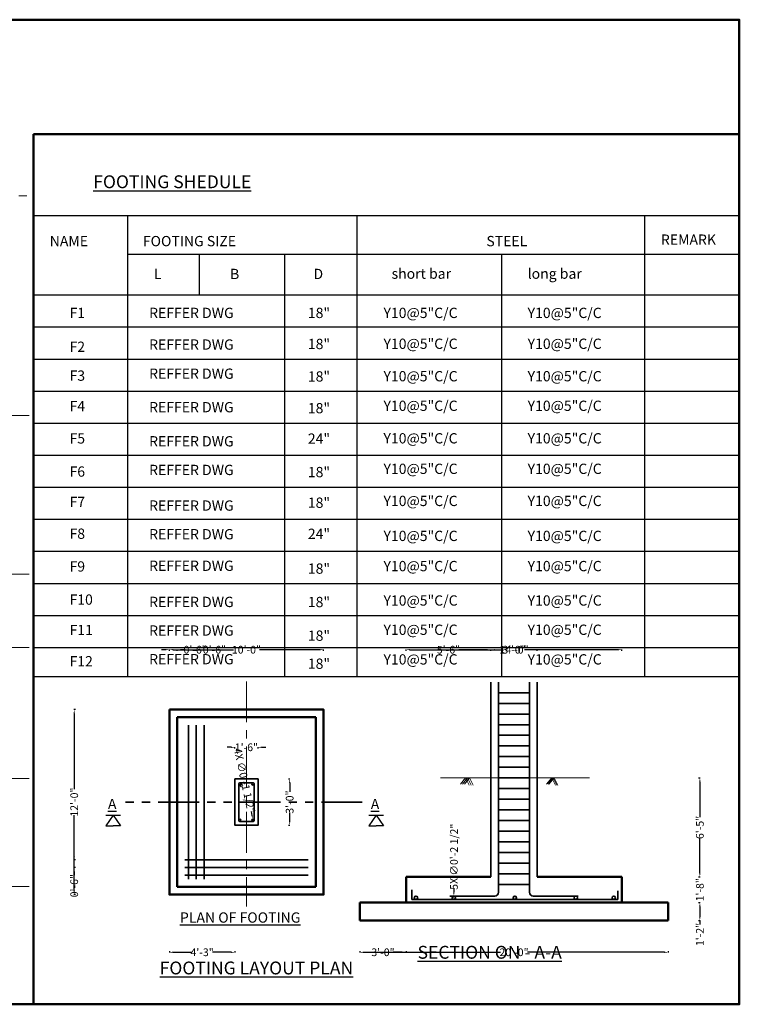
# Model space of a CAD drawing. Units: inches. Extents: x -114 to 953, y -626 to 140.
# Tile 3 of 3: x 393 to 953, y -626 to 140. Entities that reach past the tile are written whole.
import ezdxf

# ---------------------------------------------------------------- set-up
doc = ezdxf.new("R2010")
doc.units = ezdxf.units.IN
doc.header["$MEASUREMENT"] = 0
doc.linetypes.add('CENTER', pattern=[50.8, 31.75, -6.35, 6.35, -6.35])
doc.linetypes.add('PHANTOM', pattern=[63.5, 31.75, -6.35, 6.35, -6.35, 6.35, -6.35])
for name, color, linetype, lineweight in [('C-TOPO', 8, 'Continuous', 18), ('S-ANNO-DIMS', 2, 'Continuous', 25), ('S-ANNO-SCHD', 7, 'Continuous', 25), ('S-ANNO-SYMB', 3, 'Continuous', 25), ('S-ANNO-TEXT', 3, 'Continuous', 25), ('S-ANNO-TTLB', 7, 'Continuous', 50), ('S-COLS', 4, 'Continuous', 35), ('S-FNDN', 7, 'Continuous', 50), ('S-GRID', 1, 'CENTER', 18), ('S-REIN', 1, 'Continuous', 35), ('S-SECT', 6, 'PHANTOM', 35)]:
    doc.layers.add(name, color=color, linetype=linetype, lineweight=lineweight)
doc.styles.get("Standard").update_dxf_attribs({"font": 'arial.ttf'})
doc.dimstyles.get("Standard").update_dxf_attribs({"dimtxt": 6, "dimasz": 3, "dimexe": 0.18, "dimexo": 0.0625, "dimgap": 0.09, "dimtad": 0, "dimzin": 0, "dimdsep": 46, "dimlunit": 4, "dimtxsty": 'Standard', "dimcen": 0.09, "dimclrd": 256, "dimclrt": 6, "dimadec": 0, "dimazin": 0, "dimtfac": 6, "dimtofl": 0, "dimtmove": 0, "dimatfit": 3, "dimfxl": 1, "dimfxlon": 1, "dimtolj": 1, "dimtzin": 0, "dimarcsym": 0})

# ---------------------------------------------------------------- blocks, each defined once
blk = doc.blocks.new('SECTION-MARK')
for p, q in [((664.65, -479.21), (676.15, -479.21)), ((670.4, -479.21), (664.65, -487.36)), ((670.4, -479.21), (676.15, -487.36)), ((664.65, -487.36), (670.4, -487.36)), ((676.15, -487.36), (670.4, -487.36))]:
    blk.add_line(p, q)
blk = doc.blocks.new('*D64')
at = {"layer": 'Defpoints', "color": 0, "transparency": 16777216}
for p in [(629.47, -350.34), (509.47, -396.96), (629.47, -396.96)]:
    blk.add_point(p, dxfattribs=at)
at = {"layer": 'S-ANNO-DIMS', "color": 0, "lineweight": -2, "transparency": 16777216}
for p, q in [((509.47, -351.34), (509.47, -350.16)), ((629.47, -351.34), (629.47, -350.16))]:
    blk.add_line(p, q, dxfattribs=at)
at = {"layer": 'S-ANNO-DIMS', "lineweight": -2, "transparency": 16777216}
for p, q in [((512.47, -350.34), (559.36, -350.34)), ((626.47, -350.34), (579.58, -350.34))]:
    blk.add_line(p, q, dxfattribs=at)
at = {"layer": 'S-ANNO-DIMS', "transparency": 16777216}
for points in [[(512.47, -349.84), (512.47, -350.84), (509.47, -350.34)], [(626.47, -349.84), (626.47, -350.84), (629.47, -350.34)]]:
    blk.add_solid(points, dxfattribs=at)
at = {"layer": 'S-ANNO-DIMS', "color": 6, "transparency": 16777216, "insert": (569.47, -350.34), "char_height": 6, "attachment_point": 5}
blk.add_mtext('\\A1;10\'-0"', dxfattribs=at)
blk = doc.blocks.new('*D65')
at = {"layer": 'Defpoints', "color": 0, "transparency": 16777216}
for p in [(509.47, -396.96), (435.43, -540.96), (509.47, -540.96)]:
    blk.add_point(p, dxfattribs=at)
at = {"layer": 'S-ANNO-DIMS', "color": 0, "lineweight": -2, "transparency": 16777216}
for p, q in [((436.43, -396.96), (435.25, -396.96)), ((436.43, -540.96), (435.25, -540.96))]:
    blk.add_line(p, q, dxfattribs=at)
at = {"layer": 'S-ANNO-DIMS', "lineweight": -2, "transparency": 16777216}
for p, q in [((435.43, -399.96), (435.43, -458.85)), ((435.43, -537.96), (435.43, -479.07))]:
    blk.add_line(p, q, dxfattribs=at)
at = {"layer": 'S-ANNO-DIMS', "transparency": 16777216}
for points in [[(434.93, -399.96), (435.93, -399.96), (435.43, -396.96)], [(434.93, -537.96), (435.93, -537.96), (435.43, -540.96)]]:
    blk.add_solid(points, dxfattribs=at)
at = {"layer": 'S-ANNO-DIMS', "color": 6, "transparency": 16777216, "insert": (435.43, -468.96), "char_height": 6, "attachment_point": 5, "rotation": 90}
blk.add_mtext('\\A1;12\'-0"', dxfattribs=at)
blk = doc.blocks.new('*D66')
at = {"layer": 'Defpoints', "color": 0, "transparency": 16777216}
for p in [(515.47, -350.34), (509.47, -396.96), (515.47, -402.96)]:
    blk.add_point(p, dxfattribs=at)
at = {"layer": 'S-ANNO-DIMS', "lineweight": -2, "transparency": 16777216}
for p, q in [((506.47, -350.34), (503.47, -350.34)), ((518.47, -350.34), (521.47, -350.34))]:
    blk.add_line(p, q, dxfattribs=at)
at = {"layer": 'S-ANNO-DIMS', "color": 0, "lineweight": -2, "transparency": 16777216}
for p, q in [((509.47, -351.34), (509.47, -350.16)), ((515.47, -351.34), (515.47, -350.16))]:
    blk.add_line(p, q, dxfattribs=at)
at = {"layer": 'S-ANNO-DIMS', "transparency": 16777216}
for points in [[(506.47, -349.84), (506.47, -350.84), (509.47, -350.34)], [(518.47, -349.84), (518.47, -350.84), (515.47, -350.34)]]:
    blk.add_solid(points, dxfattribs=at)
at = {"layer": 'S-ANNO-DIMS', "color": 6, "transparency": 16777216, "insert": (529.54, -350.34), "char_height": 6, "attachment_point": 5}
blk.add_mtext('\\A1;0\'-6"', dxfattribs=at)
blk = doc.blocks.new('*D67')
at = {"layer": 'Defpoints', "color": 0, "transparency": 16777216}
for p in [(578.470542, -426.309234), (560.470542, -450.959234), (578.470542, -450.959234)]:
    blk.add_point(p, dxfattribs=at)
at = {"layer": 'S-ANNO-DIMS', "lineweight": -2, "transparency": 16777216}
for p, q in [((557.470542, -426.309234), (554.470542, -426.309234)), ((581.470542, -426.309234), (584.470542, -426.309234))]:
    blk.add_line(p, q, dxfattribs=at)
at = {"layer": 'S-ANNO-DIMS', "color": 0, "lineweight": -2, "transparency": 16777216}
for p, q in [((560.470542, -427.309234), (560.470542, -426.129234)), ((578.470542, -427.309234), (578.470542, -426.129234))]:
    blk.add_line(p, q, dxfattribs=at)
at = {"layer": 'S-ANNO-DIMS', "transparency": 16777216}
for points in [[(557.470542, -425.809234), (557.470542, -426.809234), (560.470542, -426.309234)], [(581.470542, -425.809234), (581.470542, -426.809234), (578.470542, -426.309234)]]:
    blk.add_solid(points, dxfattribs=at)
at = {"layer": 'S-ANNO-DIMS', "color": 6, "transparency": 16777216, "insert": (569.470542, -426.309234), "char_height": 6, "attachment_point": 5}
blk.add_mtext('\\A1;1\'-6"', dxfattribs=at)
blk = doc.blocks.new('*D68')
at = {"layer": 'Defpoints', "color": 0, "transparency": 16777216}
for p in [(578.47, -450.96), (578.47, -486.96), (603.12, -486.96)]:
    blk.add_point(p, dxfattribs=at)
at = {"layer": 'S-ANNO-DIMS', "color": 0, "lineweight": -2, "transparency": 16777216}
for p, q in [((602.12, -450.96), (603.3, -450.96)), ((602.12, -486.96), (603.3, -486.96))]:
    blk.add_line(p, q, dxfattribs=at)
at = {"layer": 'S-ANNO-DIMS', "lineweight": -2, "transparency": 16777216}
for p, q in [((603.12, -453.96), (603.12, -460.9)), ((603.12, -483.96), (603.12, -477.02))]:
    blk.add_line(p, q, dxfattribs=at)
at = {"layer": 'S-ANNO-DIMS', "transparency": 16777216}
for points in [[(602.62, -453.96), (603.62, -453.96), (603.12, -450.96)], [(602.62, -483.96), (603.62, -483.96), (603.12, -486.96)]]:
    blk.add_solid(points, dxfattribs=at)
at = {"layer": 'S-ANNO-DIMS', "color": 6, "transparency": 16777216, "insert": (603.12, -468.96), "char_height": 6, "attachment_point": 5, "rotation": 90}
blk.add_mtext('\\A1;3\'-0"', dxfattribs=at)
blk = doc.blocks.new('*D69')
at = {"layer": 'Defpoints', "color": 0, "transparency": 16777216}
for p in [(560.47, -486.96), (509.47, -540.96), (560.47, -585.86)]:
    blk.add_point(p, dxfattribs=at)
at = {"layer": 'S-ANNO-DIMS', "color": 0, "lineweight": -2, "transparency": 16777216}
for p, q in [((509.47, -584.86), (509.47, -586.04)), ((560.47, -584.86), (560.47, -586.04))]:
    blk.add_line(p, q, dxfattribs=at)
at = {"layer": 'S-ANNO-DIMS', "lineweight": -2, "transparency": 16777216}
for p, q in [((512.47, -585.86), (526.79, -585.86)), ((557.47, -585.86), (543.16, -585.86))]:
    blk.add_line(p, q, dxfattribs=at)
at = {"layer": 'S-ANNO-DIMS', "transparency": 16777216}
for points in [[(512.47, -585.36), (512.47, -586.36), (509.47, -585.86)], [(557.47, -585.36), (557.47, -586.36), (560.47, -585.86)]]:
    blk.add_solid(points, dxfattribs=at)
at = {"layer": 'S-ANNO-DIMS', "color": 6, "transparency": 16777216, "insert": (534.97, -585.86), "char_height": 6, "attachment_point": 5}
blk.add_mtext('\\A1;4\'-3"', dxfattribs=at)
blk = doc.blocks.new('*D70')
at = {"layer": 'Defpoints', "color": 0, "transparency": 16777216}
for p in [(530.47, -350.34), (524.47, -408.96), (530.47, -408.96)]:
    blk.add_point(p, dxfattribs=at)
at = {"layer": 'S-ANNO-DIMS', "lineweight": -2, "transparency": 16777216}
for p, q in [((521.47, -350.34), (518.47, -350.34)), ((533.47, -350.34), (536.47, -350.34))]:
    blk.add_line(p, q, dxfattribs=at)
at = {"layer": 'S-ANNO-DIMS', "color": 0, "lineweight": -2, "transparency": 16777216}
for p, q in [((524.47, -351.34), (524.47, -350.16)), ((530.47, -351.34), (530.47, -350.16))]:
    blk.add_line(p, q, dxfattribs=at)
at = {"layer": 'S-ANNO-DIMS', "transparency": 16777216}
for points in [[(521.47, -349.84), (521.47, -350.84), (524.47, -350.34)], [(533.47, -349.84), (533.47, -350.84), (530.47, -350.34)]]:
    blk.add_solid(points, dxfattribs=at)
at = {"layer": 'S-ANNO-DIMS', "color": 6, "transparency": 16777216, "insert": (544.54, -350.34), "char_height": 6, "attachment_point": 5}
blk.add_mtext('\\A1;0\'-6"', dxfattribs=at)
blk = doc.blocks.new('*D71')
at = {"layer": 'Defpoints', "color": 0, "transparency": 16777216}
for p in [(435.43, -519.96), (521.47, -513.96), (521.47, -519.96)]:
    blk.add_point(p, dxfattribs=at)
at = {"layer": 'S-ANNO-DIMS', "lineweight": -2, "transparency": 16777216}
for p, q in [((435.43, -510.96), (435.43, -507.96)), ((435.43, -522.96), (435.43, -525.96))]:
    blk.add_line(p, q, dxfattribs=at)
at = {"layer": 'S-ANNO-DIMS', "color": 0, "lineweight": -2, "transparency": 16777216}
for p, q in [((436.43, -513.96), (435.25, -513.96)), ((436.43, -519.96), (435.25, -519.96))]:
    blk.add_line(p, q, dxfattribs=at)
at = {"layer": 'S-ANNO-DIMS', "transparency": 16777216}
for points in [[(434.93, -510.96), (435.93, -510.96), (435.43, -513.96)], [(434.93, -522.96), (435.93, -522.96), (435.43, -519.96)]]:
    blk.add_solid(points, dxfattribs=at)
at = {"layer": 'S-ANNO-DIMS', "color": 6, "transparency": 16777216, "insert": (435.43, -534.02), "char_height": 6, "attachment_point": 5, "rotation": 90}
blk.add_mtext('\\A1;0\'-6"', dxfattribs=at)
blk = doc.blocks.new('*D72')
at = {"layer": 'Defpoints', "color": 0, "transparency": 16777216}
for p in [(657.72, -561.21), (897.72, -561.21), (897.72, -585.86)]:
    blk.add_point(p, dxfattribs=at)
at = {"layer": 'S-ANNO-DIMS', "color": 0, "lineweight": -2, "transparency": 16777216}
for p, q in [((657.72, -584.86), (657.72, -586.04)), ((897.72, -584.86), (897.72, -586.04))]:
    blk.add_line(p, q, dxfattribs=at)
at = {"layer": 'S-ANNO-DIMS', "lineweight": -2, "transparency": 16777216}
for p, q in [((660.72, -585.86), (767.27, -585.86)), ((894.72, -585.86), (788.17, -585.86))]:
    blk.add_line(p, q, dxfattribs=at)
at = {"layer": 'S-ANNO-DIMS', "transparency": 16777216}
for points in [[(660.72, -585.36), (660.72, -586.36), (657.72, -585.86)], [(894.72, -585.36), (894.72, -586.36), (897.72, -585.86)]]:
    blk.add_solid(points, dxfattribs=at)
at = {"layer": 'S-ANNO-DIMS', "color": 6, "transparency": 16777216, "insert": (777.72, -585.86), "char_height": 6, "attachment_point": 5}
blk.add_mtext('\\A1;20\'-0"', dxfattribs=at)
blk = doc.blocks.new('*D73')
at = {"layer": 'Defpoints', "color": 0, "transparency": 16777216}
for p in [(657.72, -547.21), (693.72, -547.21), (693.72, -585.86)]:
    blk.add_point(p, dxfattribs=at)
at = {"layer": 'S-ANNO-DIMS', "color": 0, "lineweight": -2, "transparency": 16777216}
for p, q in [((657.72, -584.86), (657.72, -586.04)), ((693.72, -584.86), (693.72, -586.04))]:
    blk.add_line(p, q, dxfattribs=at)
at = {"layer": 'S-ANNO-DIMS', "lineweight": -2, "transparency": 16777216}
for p, q in [((660.72, -585.86), (667.66, -585.86)), ((690.72, -585.86), (683.78, -585.86))]:
    blk.add_line(p, q, dxfattribs=at)
at = {"layer": 'S-ANNO-DIMS', "transparency": 16777216}
for points in [[(660.72, -585.36), (660.72, -586.36), (657.72, -585.86)], [(690.72, -585.36), (690.72, -586.36), (693.72, -585.86)]]:
    blk.add_solid(points, dxfattribs=at)
at = {"layer": 'S-ANNO-DIMS', "color": 6, "transparency": 16777216, "insert": (675.72, -585.86), "char_height": 6, "attachment_point": 5}
blk.add_mtext('\\A1;3\'-0"', dxfattribs=at)
blk = doc.blocks.new('*D74')
at = {"layer": 'Defpoints', "color": 0, "transparency": 16777216}
for p in [(861.72, -350.34), (693.72, -527.21), (861.72, -527.21)]:
    blk.add_point(p, dxfattribs=at)
at = {"layer": 'S-ANNO-DIMS', "color": 0, "lineweight": -2, "transparency": 16777216}
for p, q in [((693.72, -351.34), (693.72, -350.16)), ((861.72, -351.34), (861.72, -350.16))]:
    blk.add_line(p, q, dxfattribs=at)
at = {"layer": 'S-ANNO-DIMS', "lineweight": -2, "transparency": 16777216}
for p, q in [((696.72, -350.34), (767.61, -350.34)), ((858.72, -350.34), (787.83, -350.34))]:
    blk.add_line(p, q, dxfattribs=at)
at = {"layer": 'S-ANNO-DIMS', "transparency": 16777216}
for points in [[(696.72, -349.84), (696.72, -350.84), (693.72, -350.34)], [(858.72, -349.84), (858.72, -350.84), (861.72, -350.34)]]:
    blk.add_solid(points, dxfattribs=at)
at = {"layer": 'S-ANNO-DIMS', "color": 6, "transparency": 16777216, "insert": (777.72, -350.34), "char_height": 6, "attachment_point": 5}
blk.add_mtext('\\A1;14\'-0"', dxfattribs=at)
blk = doc.blocks.new('*D75')
at = {"layer": 'Defpoints', "color": 0, "transparency": 16777216}
for p in [(897.72, -547.21), (897.72, -561.21), (922.37, -561.21)]:
    blk.add_point(p, dxfattribs=at)
at = {"layer": 'S-ANNO-DIMS', "color": 0, "lineweight": -2, "transparency": 16777216}
for p, q in [((921.37, -547.21), (922.55, -547.21)), ((921.37, -561.21), (922.55, -561.21))]:
    blk.add_line(p, q, dxfattribs=at)
at = {"layer": 'S-ANNO-DIMS', "lineweight": -2, "transparency": 16777216}
for p, q in [((922.37, -550.21), (922.37, -558.21)), ((922.37, -561.21), (922.37, -564.21))]:
    blk.add_line(p, q, dxfattribs=at)
at = {"layer": 'S-ANNO-DIMS', "transparency": 16777216}
for points in [[(921.87, -550.21), (922.87, -550.21), (922.37, -547.21)], [(921.87, -558.21), (922.87, -558.21), (922.37, -561.21)]]:
    blk.add_solid(points, dxfattribs=at)
at = {"layer": 'S-ANNO-DIMS', "color": 6, "transparency": 16777216, "insert": (922.37, -571.99), "char_height": 6, "attachment_point": 5, "rotation": 90}
blk.add_mtext('\\A1;1\'-2"', dxfattribs=at)
blk = doc.blocks.new('*D76')
at = {"layer": 'Defpoints', "color": 0, "transparency": 16777216}
for p in [(861.721337, -527.205723), (861.721337, -547.205723), (922.371337, -547.205723)]:
    blk.add_point(p, dxfattribs=at)
at = {"layer": 'S-ANNO-DIMS', "color": 0, "lineweight": -2, "transparency": 16777216}
for p, q in [((921.371337, -527.205723), (922.551337, -527.205723)), ((921.371337, -547.205723), (922.551337, -547.205723))]:
    blk.add_line(p, q, dxfattribs=at)
at = {"layer": 'S-ANNO-DIMS', "lineweight": -2, "transparency": 16777216}
for p, q in [((922.371337, -524.205723), (922.371337, -521.205723)), ((922.371337, -550.205723), (922.371337, -553.205723))]:
    blk.add_line(p, q, dxfattribs=at)
at = {"layer": 'S-ANNO-DIMS', "transparency": 16777216}
for points in [[(921.871337, -524.205723), (922.871337, -524.205723), (922.371337, -527.205723)], [(921.871337, -550.205723), (922.871337, -550.205723), (922.371337, -547.205723)]]:
    blk.add_solid(points, dxfattribs=at)
at = {"layer": 'S-ANNO-DIMS', "color": 6, "transparency": 16777216, "insert": (922.371337, -537.205723), "char_height": 6, "attachment_point": 5, "rotation": 90}
blk.add_mtext('\\A1;1\'-8"', dxfattribs=at)
blk = doc.blocks.new('*D77')
at = {"layer": 'Defpoints', "color": 0, "transparency": 16777216}
for p in [(795.72, -350.34), (759.72, -375.52), (795.72, -375.52)]:
    blk.add_point(p, dxfattribs=at)
at = {"layer": 'S-ANNO-DIMS', "color": 0, "lineweight": -2, "transparency": 16777216}
for p, q in [((759.72, -351.34), (759.72, -350.16)), ((795.72, -351.34), (795.72, -350.16))]:
    blk.add_line(p, q, dxfattribs=at)
at = {"layer": 'S-ANNO-DIMS', "lineweight": -2, "transparency": 16777216}
for p, q in [((762.72, -350.34), (769.66, -350.34)), ((792.72, -350.34), (785.78, -350.34))]:
    blk.add_line(p, q, dxfattribs=at)
at = {"layer": 'S-ANNO-DIMS', "transparency": 16777216}
for points in [[(762.72, -349.84), (762.72, -350.84), (759.72, -350.34)], [(792.72, -349.84), (792.72, -350.84), (795.72, -350.34)]]:
    blk.add_solid(points, dxfattribs=at)
at = {"layer": 'S-ANNO-DIMS', "color": 6, "transparency": 16777216, "insert": (777.72, -350.34), "char_height": 6, "attachment_point": 5}
blk.add_mtext('\\A1;3\'-0"', dxfattribs=at)
blk = doc.blocks.new('*D78')
at = {"layer": 'Defpoints', "color": 0, "transparency": 16777216}
for p in [(759.72, -350.34), (693.72, -527.21), (759.72, -527.21)]:
    blk.add_point(p, dxfattribs=at)
at = {"layer": 'S-ANNO-DIMS', "color": 0, "lineweight": -2, "transparency": 16777216}
for p, q in [((693.72, -351.34), (693.72, -350.16)), ((759.72, -351.34), (759.72, -350.16))]:
    blk.add_line(p, q, dxfattribs=at)
at = {"layer": 'S-ANNO-DIMS', "lineweight": -2, "transparency": 16777216}
for p, q in [((696.72, -350.34), (718.66, -350.34)), ((756.72, -350.34), (734.79, -350.34))]:
    blk.add_line(p, q, dxfattribs=at)
at = {"layer": 'S-ANNO-DIMS', "transparency": 16777216}
for points in [[(696.72, -349.84), (696.72, -350.84), (693.72, -350.34)], [(756.72, -349.84), (756.72, -350.84), (759.72, -350.34)]]:
    blk.add_solid(points, dxfattribs=at)
at = {"layer": 'S-ANNO-DIMS', "color": 6, "transparency": 16777216, "insert": (726.72, -350.34), "char_height": 6, "attachment_point": 5}
blk.add_mtext('\\A1;5\'-6"', dxfattribs=at)
blk = doc.blocks.new('*D79')
at = {"layer": 'Defpoints', "color": 0, "transparency": 16777216}
for p in [(836.59, -450.18), (861.72, -527.21), (922.37, -527.21)]:
    blk.add_point(p, dxfattribs=at)
at = {"layer": 'S-ANNO-DIMS', "color": 0, "lineweight": -2, "transparency": 16777216}
for p, q in [((921.37, -450.18), (922.55, -450.18)), ((921.37, -527.21), (922.55, -527.21))]:
    blk.add_line(p, q, dxfattribs=at)
at = {"layer": 'S-ANNO-DIMS', "lineweight": -2, "transparency": 16777216}
for p, q in [((922.37, -453.18), (922.37, -480.61)), ((922.37, -524.21), (922.37, -496.77))]:
    blk.add_line(p, q, dxfattribs=at)
at = {"layer": 'S-ANNO-DIMS', "transparency": 16777216}
for points in [[(921.87, -453.18), (922.87, -453.18), (922.37, -450.18)], [(921.87, -524.21), (922.87, -524.21), (922.37, -527.21)]]:
    blk.add_solid(points, dxfattribs=at)
at = {"layer": 'S-ANNO-DIMS', "color": 6, "transparency": 16777216, "insert": (922.37, -488.69), "char_height": 6, "attachment_point": 5, "rotation": 90}
blk.add_mtext('\\A1;6\'-5"', dxfattribs=at)
blk = doc.blocks.new('*D80')
at = {"layer": 'Defpoints', "color": 0, "transparency": 16777216}
for p in [(730.9, -542.07), (730.89, -544.71)]:
    blk.add_point(p, dxfattribs=at)
at = {"layer": 'S-ANNO-DIMS', "lineweight": -2, "transparency": 16777216}
blk.add_line((730.92, -536.07), (730.91, -539.07), dxfattribs=at)
at = {"layer": 'S-ANNO-DIMS', "color": 0, "lineweight": -2, "transparency": 16777216}
for p, q in [((730.81, -543.39), (730.99, -543.39)), ((730.9, -543.48), (730.9, -543.3))]:
    blk.add_line(p, q, dxfattribs=at)
at = {"layer": 'S-ANNO-DIMS', "transparency": 16777216}
blk.add_solid([(730.41, -539.07), (731.41, -539.08), (730.9, -542.07)], dxfattribs=at)
at = {"layer": 'S-ANNO-DIMS', "color": 6, "transparency": 16777216, "insert": (731.01, -511.47), "char_height": 6, "attachment_point": 5, "rotation": 89.79463}
blk.add_mtext('\\A1;5X ∅0\'-2 1/2"', dxfattribs=at)
blk = doc.blocks.new('*D81')
at = {"layer": 'Defpoints', "color": 0, "transparency": 16777216}
for p in [(574.42, -482.25), (574.79, -483.94)]:
    blk.add_point(p, dxfattribs=at)
at = {"layer": 'S-ANNO-DIMS', "lineweight": -2, "transparency": 16777216}
blk.add_line((573.16, -476.38), (573.79, -479.32), dxfattribs=at)
at = {"layer": 'S-ANNO-DIMS', "color": 0, "lineweight": -2, "transparency": 16777216}
for p, q in [((574.52, -483.1), (574.7, -483.1)), ((574.61, -483.19), (574.61, -483.01))]:
    blk.add_line(p, q, dxfattribs=at)
at = {"layer": 'S-ANNO-DIMS', "transparency": 16777216}
blk.add_solid([(574.28, -479.21), (573.3, -479.42), (574.42, -482.25)], dxfattribs=at)
at = {"layer": 'S-ANNO-DIMS', "color": 6, "transparency": 16777216, "insert": (567.96, -452.21), "char_height": 6, "attachment_point": 5, "rotation": 282.14454}
blk.add_mtext('\\A1;4X ∅0\'-1 1/2"', dxfattribs=at)

msp = doc.modelspace()

# ---------------------------------------------------------------- linework, layer by layer
at = {"layer": 'C-TOPO'}
for p, q in [((765.721, -450.18), (720.576, -450.18)), ((740.037, -450.18), (736.031, -454.899)), ((741.517, -450.18), (737.51, -454.899)), ((743.149, -450.18), (739.142, -454.899)), ((740.037, -450.18), (742.876, -455.899)), ((741.517, -450.18), (744.355, -455.899)), ((743.149, -450.18), (745.987, -455.899)), ((789.721, -450.18), (836.59, -450.18)), ((807.104, -450.18), (803.097, -454.899)), ((808.197, -450.18), (804.19, -454.899)), ((808.923, -450.18), (804.917, -454.899)), ((807.104, -450.18), (809.942, -455.899)), ((808.197, -450.18), (811.035, -455.899)), ((808.923, -450.18), (811.761, -455.899))]:
    msp.add_line(p, q, dxfattribs=at)
at = {"layer": 'S-ANNO-SCHD'}
for p, q in [((476.825, -12.309), (476.825, -371.554)), ((655.403, -12.309), (655.403, -371.554)), ((879.341, -12.309), (879.341, -371.554)), ((476.825, -42.59), (953.065, -42.59)), ((532.591, -42.59), (532.591, -74.219)), ((599.019, -42.59), (599.019, -371.554)), ((768.005, -42.59), (768.005, -371.554)), ((403.662, -74.219), (953.065, -74.219)), ((403.662, -99.164), (953.065, -99.164)), ((403.662, -124.109), (953.065, -124.109)), ((403.662, -149.054), (953.065, -149.054)), ((403.662, -173.999), (953.065, -173.999)), ((403.662, -198.944), (953.065, -198.944)), ((403.662, -223.889), (953.065, -223.889)), ((403.662, -248.833), (953.065, -248.833)), ((403.662, -273.778), (953.065, -273.778)), ((403.662, -298.723), (953.065, -298.723)), ((403.662, -323.668), (953.065, -323.668)), ((403.662, -348.613), (953.065, -348.613))]:
    msp.add_line(p, q, dxfattribs=at)
msp.add_lwpolyline([(953.065, -371.554), (403.662, -371.554), (403.662, -12.309), (953.065, -12.309)], dxfattribs=at)
at = {"layer": 'S-ANNO-TTLB'}
for points in [[(-86.343, 140.009), (953.065, 140.009), (953.065, -626.35), (-86.343, -626.35)], [(403.662, 50.843), (953.065, 50.843), (953.065, -626.35), (403.662, -626.35)]]:
    msp.add_lwpolyline(points, close=True, dxfattribs=at)
at = {"layer": 'S-COLS'}
for p, q in [((759.721, -527.206), (759.721, -375.516)), ((795.721, -527.206), (795.721, -375.516))]:
    msp.add_line(p, q, dxfattribs=at)
msp.add_lwpolyline([(560.471, -450.959), (578.471, -450.959), (578.471, -486.959), (560.471, -486.959)], close=True, dxfattribs=at)
at = {"layer": 'S-FNDN'}
for p, q in [((515.471, -402.959), (623.471, -402.959)), ((515.471, -534.959), (515.471, -402.959)), ((623.471, -402.959), (623.471, -534.959)), ((693.721, -547.206), (693.721, -527.206)), ((693.721, -527.206), (759.721, -527.206)), ((795.721, -527.206), (861.721, -527.206)), ((861.721, -547.206), (861.721, -527.206)), ((623.471, -534.959), (515.471, -534.959)), ((897.721, -547.206), (657.721, -547.206)), ((657.721, -547.206), (657.721, -561.206)), ((897.721, -547.206), (861.721, -547.206)), ((897.721, -556.206), (897.721, -547.206)), ((897.721, -561.206), (897.721, -556.206)), ((657.721, -561.206), (897.721, -561.206))]:
    msp.add_line(p, q, dxfattribs=at)
msp.add_lwpolyline([(509.471, -396.959), (629.471, -396.959), (629.471, -540.959), (509.471, -540.959)], close=True, dxfattribs=at)
at = {"layer": 'S-GRID'}
for p, q in [((-52.223, 2.831), (403.662, 2.831)), ((-37.867, -168.169), (403.662, -168.169)), ((-37.867, -291.669), (403.662, -291.669)), ((-37.867, -348.669), (403.662, -348.669)), ((569.471, -374.987), (569.471, -550.338)), ((-37.867, -450.669), (403.662, -450.669)), ((-37.867, -534.669), (403.662, -534.669))]:
    msp.add_line(p, q, dxfattribs=at)
at = {"layer": 'S-REIN'}
for p, q in [((765.721, -527.206), (765.721, -375.516)), ((789.721, -527.206), (789.721, -375.516)), ((765.721, -383.812), (789.721, -383.812)), ((765.721, -392.108), (789.721, -392.108)), ((765.721, -400.404), (789.721, -400.404)), ((524.471, -528.959), (524.471, -408.959)), ((530.471, -528.959), (530.471, -408.959)), ((536.471, -528.959), (536.471, -408.959)), ((765.721, -408.7), (789.721, -408.7)), ((765.721, -416.996), (789.721, -416.996)), ((765.721, -425.292), (789.721, -425.292)), ((765.721, -433.588), (789.721, -433.588)), ((765.721, -441.884), (789.721, -441.884)), ((765.721, -450.18), (789.721, -450.18)), ((563.775, -455.481), (565.66, -457.086)), ((564.938, -454.205), (566.748, -455.971)), ((765.721, -458.476), (789.721, -458.476)), ((765.721, -466.772), (789.721, -466.772)), ((765.721, -475.068), (789.721, -475.068)), ((765.721, -483.364), (789.721, -483.364)), ((765.721, -491.66), (789.721, -491.66)), ((765.721, -499.956), (789.721, -499.956)), ((765.721, -508.252), (789.721, -508.252)), ((617.471, -513.959), (521.471, -513.959)), ((617.471, -519.959), (521.471, -519.959)), ((765.721, -516.548), (789.721, -516.548)), ((617.471, -525.959), (521.471, -525.959)), ((765.721, -524.844), (789.721, -524.844)), ((765.721, -527.206), (765.721, -539.074)), ((789.721, -527.206), (789.721, -539.074)), ((765.721, -533.14), (789.721, -533.14)), ((698.218, -544.706), (698.218, -537.327)), ((762.721, -542.074), (727.691, -542.074)), ((792.721, -542.074), (827.752, -542.074)), ((858.606, -538.041), (858.606, -544.706)), ((858.606, -544.706), (698.218, -544.706))]:
    msp.add_line(p, q, dxfattribs=at)
for points in [[(563.471, -483.095), (563.471, -454.823)], [(564.335, -453.959), (574.607, -453.959)], [(575.471, -454.823), (575.471, -483.095)], [(574.607, -483.959), (564.335, -483.959)]]:
    msp.add_lwpolyline(points, dxfattribs=at)
for centre, radius in [((564.335, -454.823), 0.864), ((574.607, -454.823), 0.864), ((564.335, -483.095), 0.864), ((574.607, -483.095), 0.864), ((701.421, -543.39), 1.316), ((730.898, -543.39), 1.316), ((778.328, -543.39), 1.316), ((778.412, -543.39), 1.316), ((825.842, -543.39), 1.316), ((855.318, -543.39), 1.316)]:
    msp.add_circle(centre, radius, dxfattribs=at)
for centre, start, end in [((762.721, -539.074), 270, 0), ((792.721, -539.074), 180, 270)]:
    msp.add_arc(centre, 3, start, end, dxfattribs=at)
at = {"layer": 'S-SECT'}
msp.add_line((659.593, -468.959), (473.882, -468.959), dxfattribs=at)

# ---------------------------------------------------------------- block references
at = {"layer": 'S-ANNO-SYMB'}
for p in [(-204.57, 0), (0, 0)]:
    msp.add_blockref('SECTION-MARK', p, dxfattribs=at)

# ---------------------------------------------------------------- texts
at = {"layer": 'S-ANNO-TEXT', "attachment_point": 1}
for s, width, insert, char_height in [('{\\fArial|b1|i0|c0|p34;\\LFOOTING SHEDULE}', 171.9614, (450.242, 18.859), 10), ('{\\fArial|b1|i0|c0|p34;NAME}', 117.31259, (416.369, -28.326), 8), ('{\\fArial|b1|i0|c0|p34;FOOTING SIZE}', 117.31259, (488.85, -28.326), 8), ('{\\fArial|b1|i0|c0|p34;STEEL}', 117.31259, (756.218, -28.326), 8), ('{\\fArial|b1|i0|c0|p34;REMARK}', 117.31259, (892.058, -27.178), 8), ('{\\fArial|b1|i0|c0|p34;short bar }', 117.31259, (682.452, -53.653), 8), ('{\\fArial|b1|i0|c0|p34;long bar}', 117.31259, (788.362, -53.653), 8), ('{\\fArial|b1|i0|c0|p34;L}', 117.31259, (497.407, -53.901), 8), ('{\\fArial|b1|i0|c0|p34;B}', 117.31259, (556.713, -53.901), 8), ('{\\fArial|b1|i0|c0|p34;D}', 117.31259, (621.647, -53.901), 8), ('F1', 8, (431.793, -84.2), 8), ('REFFER DWG', 84.43388, (493.728, -84.2), 8), ('18"', 8, (617.269, -84.2), 8), ('Y10@5"C/C', 8, (676.145, -84.2), 8), ('Y10@5"C/C', 8, (788.306, -84.2), 8), ('F2', 8, (431.793, -110.554), 8), ('REFFER DWG', 84.43388, (493.728, -108.839), 8), ('18"', 8, (617.269, -108.389), 8), ('Y10@5"C/C', 8, (676.145, -108.224), 8), ('Y10@5"C/C', 8, (788.306, -108.224), 8), ('F3', 8, (431.793, -133.03), 8), ('REFFER DWG', 84.43388, (493.728, -131.514), 8), ('18"', 8, (617.269, -133.65), 8), ('Y10@5"C/C', 8, (676.145, -133.48), 8), ('Y10@5"C/C', 8, (788.306, -133.48), 8), ('F4', 8, (431.793, -156.754), 8), ('REFFER DWG', 84.43388, (493.728, -157.591), 8), ('18"', 8, (617.269, -158.341), 8), ('Y10@5"C/C', 8, (676.145, -156.497), 8), ('Y10@5"C/C', 8, (788.306, -156.497), 8), ('F5', 8, (431.793, -181.895), 8), ('24"', 8, (617.269, -182.071), 8), ('Y10@5"C/C', 8, (676.145, -181.81), 8), ('Y10@5"C/C', 8, (788.306, -181.81), 8), ('REFFER DWG', 84.43388, (493.728, -184.13), 8), ('REFFER DWG', 84.43388, (493.728, -206.427), 8), ('Y10@5"C/C', 8, (676.145, -205.554), 8), ('Y10@5"C/C', 8, (788.306, -205.554), 8), ('F6', 8, (431.793, -207.688), 8), ('18"', 8, (617.269, -208.097), 8), ('Y10@5"C/C', 8, (676.145, -230.551), 8), ('Y10@5"C/C', 8, (788.306, -230.551), 8), ('F7', 8, (431.793, -231.363), 8), ('REFFER DWG', 84.43388, (493.728, -234.153), 8), ('18"', 8, (617.269, -231.924), 8), ('F8', 8, (431.793, -256.05), 8), ('REFFER DWG', 84.43388, (493.728, -256.45), 8), ('24"', 8, (617.269, -256.139), 8), ('Y10@5"C/C', 8, (676.145, -257.766), 8), ('Y10@5"C/C', 8, (788.306, -257.766), 8), ('F9', 8, (431.793, -281.558), 8), ('REFFER DWG', 84.43388, (493.728, -281.015), 8), ('18"', 8, (617.269, -283.21), 8), ('Y10@5"C/C', 8, (676.145, -281.267), 8), ('Y10@5"C/C', 8, (788.306, -281.267), 8), ('F10', 8, (431.793, -307.351), 8), ('REFFER DWG', 84.43388, (493.728, -309.15), 8), ('18"', 8, (617.269, -309.237), 8), ('Y10@5"C/C', 8, (676.145, -308.048), 8), ('Y10@5"C/C', 8, (788.306, -308.048), 8), ('F11', 8, (431.793, -331.02), 8), ('REFFER DWG', 84.43388, (493.728, -331.447), 8), ('18"', 8, (617.269, -335.418), 8), ('Y10@5"C/C', 8, (676.145, -330.823), 8), ('Y10@5"C/C', 8, (788.306, -330.823), 8), ('F12', 8, (431.793, -355.339), 8), ('REFFER DWG', 84.43388, (493.728, -353.744), 8), ('18"', 8, (617.269, -357.234), 8), ('Y10@5"C/C', 8, (676.145, -353.877), 8), ('Y10@5"C/C', 8, (788.306, -353.877), 8), ('{\\fArial|b1|i0|c0|p34;\\LA}', 16.75606, (461.675, -466.435), 8), ('{\\fArial|b1|i0|c0|p34;\\LA}', 16.75606, (666.246, -466.435), 8), ('{\\fArial|b1|i0|c0|p34;\\LPLAN OF FOOTING}', 117.31259, (517.725, -554.805), 8), ('{\\fArial|b1|i0|c0|p34;\\LSECTION ON - A-A}', 132.49062, (702.657, -580.868), 10), ('{\\fArial|b1|i0|c0|p34;\\LFOOTING LAYOUT PLAN}', 171.9614, (501.939, -593.07), 10)]:
    msp.add_mtext_dynamic_manual_height_columns(s, width=width, gutter_width=1, heights=[0], dxfattribs=dict(at, insert=insert, char_height=char_height))

# ---------------------------------------------------------------- dimensions: what is measured, and where the dimension line sits
at = {"layer": 'S-ANNO-DIMS'}
for base, p1, p2, picture, middle in [((515.471, -350.337), (509.471, -396.959), (515.471, -402.959), '*D66', (529.535, -350.337)), ((629.471, -350.337), (509.471, -396.959), (629.471, -396.959), '*D64', (569.471, -350.337)), ((530.471, -350.337), (524.471, -408.959), (530.471, -408.959), '*D70', (544.535, -350.337)), ((861.721, -350.337), (693.721, -527.206), (861.721, -527.206), '*D74', (777.721, -350.337)), ((759.721, -350.337), (693.721, -527.206), (759.721, -527.206), '*D78', (726.721, -350.337)), ((795.721, -350.337), (759.721, -375.516), (795.721, -375.516), '*D77', (777.721, -350.337)), ((578.471, -426.309), (560.471, -450.959), (578.471, -450.959), '*D67', (569.471, -426.309)), ((560.471, -585.856), (509.471, -540.959), (560.471, -486.959), '*D69', (534.971, -585.856)), ((693.721, -585.856), (657.721, -547.206), (693.721, -547.206), '*D73', (675.721, -585.856)), ((897.721, -585.856), (657.721, -561.206), (897.721, -561.206), '*D72', (777.721, -585.856))]:
    dim = msp.add_linear_dim(base=base, p1=p1, p2=p2, dimstyle='Standard', override={"dimdec": 1, "dimlfac": 1, "dimrnd": 0, "dimzin": 1, "dimdsep": 46, "dimlunit": 4, "dimfrac": 2}, dxfattribs=at)
    dim.commit()
    dim.dimension.update_dxf_attribs({"geometry": picture, "text_midpoint": middle})
for base, p1, p2, angle, picture, middle in [((435.43, -540.959), (509.471, -396.959), (509.471, -540.959), 90, '*D65', (435.43, -468.959)), ((603.121, -486.959), (578.471, -450.959), (578.471, -486.959), 270, '*D68', (603.121, -468.959)), ((922.371, -527.206), (836.59, -450.18), (861.721, -527.206), 90, '*D79', (922.371, -488.693)), ((435.43, -519.959), (521.471, -513.959), (521.471, -519.959), 90, '*D71', (435.43, -534.024)), ((922.371, -547.206), (861.721, -527.206), (861.721, -547.206), 90, '*D76', (922.371, -537.206)), ((922.371, -561.206), (897.721, -547.206), (897.721, -561.206), 90, '*D75', (922.371, -571.988))]:
    dim = msp.add_linear_dim(base=base, p1=p1, p2=p2, angle=angle, dimstyle='Standard', override={"dimdec": 1, "dimlfac": 1, "dimrnd": 0, "dimzin": 1, "dimdsep": 46, "dimlunit": 4, "dimfrac": 2}, dxfattribs=at)
    dim.commit()
    dim.dimension.update_dxf_attribs({"geometry": picture, "text_midpoint": middle})
for p1, p2, text, picture, middle in [((574.788, -483.94), (574.425, -482.251), '4X <>', '*D81', (567.961, -452.212)), ((730.893, -544.706), (730.903, -542.074), '5X <>', '*D80', (731.012, -511.469))]:
    dim = msp.add_diameter_dim_2p(p1=p1, p2=p2, text=text, dimstyle='Standard', override={"dimdec": 1, "dimlfac": 1, "dimrnd": 0, "dimzin": 1, "dimdsep": 46, "dimlunit": 4, "dimfrac": 2}, dxfattribs=at)
    dim.commit()
    dim.dimension.update_dxf_attribs({"geometry": picture, "text_midpoint": middle, "dimtype": 163})

doc.saveas('drawing.dxf')
